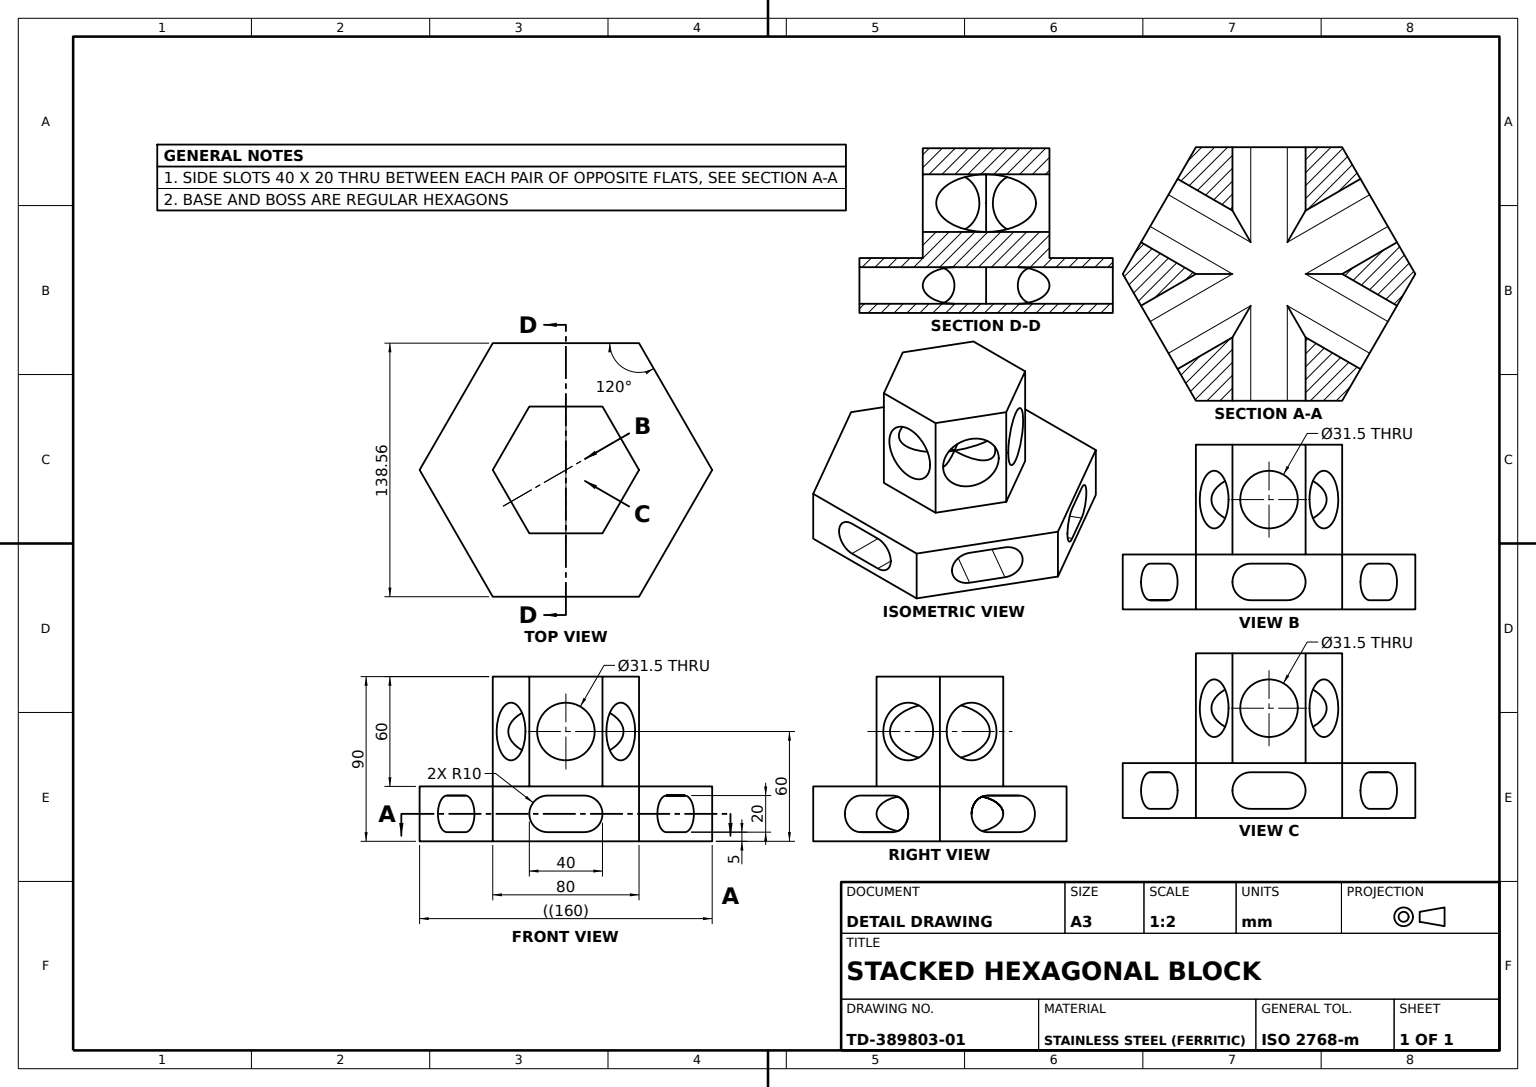
from build123d import *

# Parameters (mm, degrees)
HEX_BASE_DEPTH          = 15
SIDE_SLOT_1_20X10_DEPTH = 161.7015868
SIDE_SLOT_2_20X10_DEPTH = 176
SIDE_SLOT_3_20X10_DEPTH = 176
HEX_BOSS_DEPTH          = 60
CROSS_HOLE_1_SKETCH_R   = 15.75
CROSS_HOLE_1_31_5_DEPTH = 152.079449297
CROSS_HOLE_2_SKETCH_R   = 15.75
CROSS_HOLE_2_31_5_DEPTH = 159.823801743
CROSS_HOLE_3_SKETCH_R   = 15.75
CROSS_HOLE_3_31_5_DEPTH = 159.823801743


with BuildPart() as part:
    # Hex Base Sketch → Hex Base (new, symmetric)
    with BuildSketch(Plane(origin=(0, 0, 0), x_dir=(1, 0, 0), z_dir=(0, 1, 0))):
        Polygon((69.282032303, -40), (69.282032303, 40), (0, 80), (-69.282032303, 40), (-69.282032303, -40), (0, -80), align=None)
    extrude(amount=HEX_BASE_DEPTH, both=True)

    # Side Slot 1 Sketch → Side Slot 1 20x10 (cut, through all)
    with BuildSketch(Plane.ZY.offset(69.282032303)):
        with BuildLine():
            Line((-10, 10), (10, 10))
            ThreePointArc((10, 10), (20, 0), (10, -10))
            Line((10, -10), (-10, -10))
            ThreePointArc((-10, -10), (-20, 0), (-10, 10))
        make_face()
    extrude(amount=-SIDE_SLOT_1_20X10_DEPTH, mode=Mode.SUBTRACT)

    # Side Slot 2 Sketch → Side Slot 2 20x10 (cut, through all)
    with BuildSketch(Plane(origin=(34.641016151, 0, -60), x_dir=(-0.8660254037844386, 0, -0.5000000000000003), z_dir=(0.5000000000000002, 0, -0.8660254037844385))):
        with BuildLine():
            Line((-10, 10), (10, 10))
            ThreePointArc((10, 10), (20, 0), (10, -10))
            Line((10, -10), (-10, -10))
            ThreePointArc((-10, -10), (-20, 0), (-10, 10))
        make_face()
    extrude(amount=-SIDE_SLOT_2_20X10_DEPTH, mode=Mode.SUBTRACT)

    # Side Slot 3 Sketch → Side Slot 3 20x10 (cut, through all)
    with BuildSketch(Plane(origin=(-34.641016151, 0, -60), x_dir=(-0.8660254037844388, 0, 0.49999999999999983), z_dir=(-0.4999999999999998, 0, -0.8660254037844387))):
        with BuildLine():
            Line((-10, 10), (10, 10))
            ThreePointArc((10, 10), (20, 0), (10, -10))
            Line((10, -10), (-10, -10))
            ThreePointArc((-10, -10), (-20, 0), (-10, 10))
        make_face()
    extrude(amount=-SIDE_SLOT_3_20X10_DEPTH, mode=Mode.SUBTRACT)

    # Hex Boss Sketch → Hex Boss (add)
    with BuildSketch(Plane(origin=(0, 15, 0), x_dir=(1, 0, 0), z_dir=(0, 1, 0))):
        Polygon((34.641016151, -20), (34.641016151, 20), (0, 40), (-34.641016151, 20), (-34.641016151, -20), (0, -40), align=None)
    extrude(amount=HEX_BOSS_DEPTH)

    # Cross Hole 1 Sketch → Cross Hole 1 Ø31.5 (cut, through all)
    with BuildSketch(Plane(origin=(34.641016151, 0, 0), x_dir=(0, 0, -1), z_dir=(1, 0, 0))):
        with Locations((0, 45)):
            Circle(CROSS_HOLE_1_SKETCH_R)
    extrude(amount=-CROSS_HOLE_1_31_5_DEPTH, mode=Mode.SUBTRACT)

    # Cross Hole 2 Sketch → Cross Hole 2 Ø31.5 (cut, through all)
    with BuildSketch(Plane(origin=(17.320508076, 0, -30), x_dir=(-0.8660254037844384, 0, -0.5000000000000004), z_dir=(0.5000000000000004, 0, -0.8660254037844384))):
        with Locations((0, 45)):
            Circle(CROSS_HOLE_2_SKETCH_R)
    extrude(amount=-CROSS_HOLE_2_31_5_DEPTH, mode=Mode.SUBTRACT)

    # Cross Hole 3 Sketch → Cross Hole 3 Ø31.5 (cut, through all)
    with BuildSketch(Plane(origin=(17.320508076, 0, 30), x_dir=(0.8660254037844388, 0, -0.4999999999999997), z_dir=(0.4999999999999997, 0, 0.8660254037844388))):
        with Locations((0, 45)):
            Circle(CROSS_HOLE_3_SKETCH_R)
    extrude(amount=-CROSS_HOLE_3_31_5_DEPTH, mode=Mode.SUBTRACT)


solid = part.part
